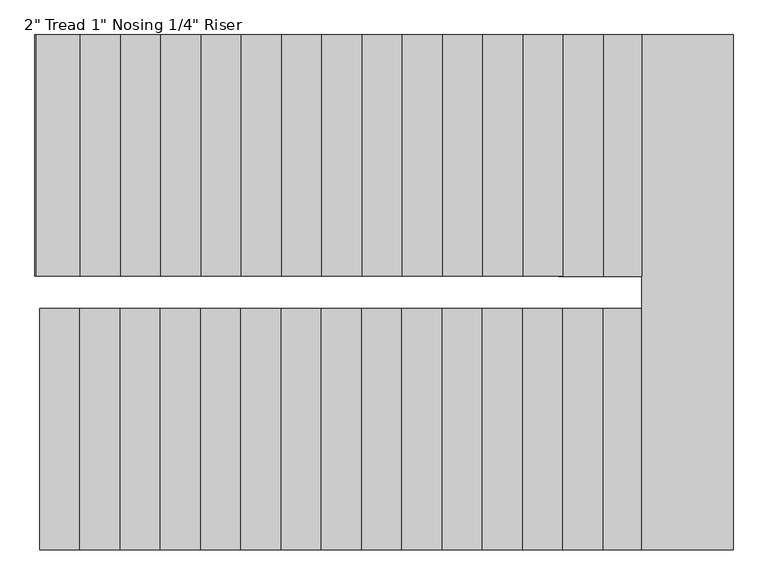
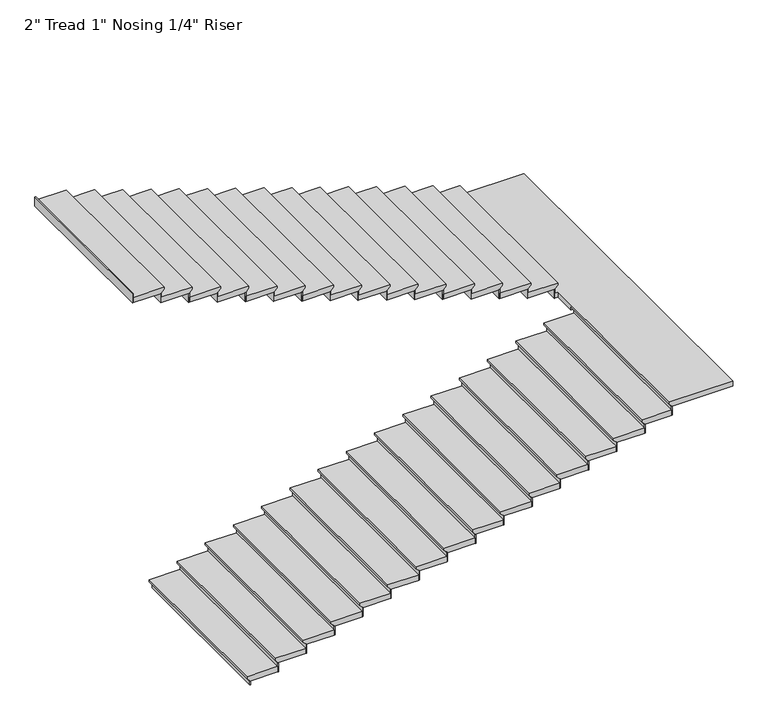
"""IFC4 building model written with IfcOpenShell, lengths in millimetres: stair flight geometry."""

from ifc_helpers import new_model, si_unit, origin, place, context, project, spatial, faceted_brep, source, transform, mapped, element, save


def stair_flight_62363484(model_context):
    return source(origin(), model_context, "Body", "Brep", [
        faceted_brep([(1449.3932247, -2065.2659014, 66.675), (1449.3932247, -2065.2659014, 85.725), (1449.3932247, -541.2659014, 85.725), (1449.3932247, -541.2659014, 66.675), (1474.7932247, -2065.2659014, 41.275), (1474.7932247, -541.2659014, 41.275), (1726.3621616, -2065.2659014, 85.725), (1726.3621616, -541.2659014, 85.725), (1474.7932247, -541.2659014, 34.925), (1726.3621616, -541.2659014, 34.925), (1726.3621616, -2065.2659014, 34.925), (1474.7932247, -2065.2659014, 34.925)], [[[0, 1, 2, 3]], [[4, 0, 3, 5]], [[2, 1, 6, 7]], [[8, 9, 10, 11]], [[2, 7, 9, 8, 5, 3]], [[8, 11, 4, 5]], [[6, 1, 0, 4, 11, 10]], [[7, 6, 10, 9]]]),
        faceted_brep([(1474.7932247, -2065.2659014, 34.925), (1474.7932247, -2065.2659014, 0.0), (1481.1432247, -2065.2659014, 0.0), (1481.1432247, -2065.2659014, 34.925), (1474.7932247, -541.2659014, 34.925), (1481.1432247, -541.2659014, 34.925), (1481.1432247, -541.2659014, 0.0), (1474.7932247, -541.2659014, 0.0)], [[[0, 1, 2, 3]], [[4, 5, 6, 7]], [[1, 0, 4, 7]], [[2, 1, 7, 6]], [[3, 2, 6, 5]], [[0, 3, 5, 4]]]),
        faceted_brep([(1726.3621616, -2065.2659014, 120.65), (1726.3621616, -2065.2659014, 34.925), (1732.7121616, -2065.2659014, 34.925), (1732.7121616, -2065.2659014, 120.65), (1726.3621616, -541.2659014, 120.65), (1732.7121616, -541.2659014, 120.65), (1732.7121616, -541.2659014, 34.925), (1726.3621616, -541.2659014, 34.925)], [[[0, 1, 2, 3]], [[4, 5, 6, 7]], [[1, 0, 4, 7]], [[2, 1, 7, 6]], [[3, 2, 6, 5]], [[0, 3, 5, 4]]]),
        faceted_brep([(1700.9621616, -541.2659014, 171.45), (1700.9621616, -2065.2659014, 171.45), (1980.3621616, -2065.2659014, 171.45), (1980.3621616, -541.2659014, 171.45), (1726.3621616, -541.2659014, 120.65), (1980.3621616, -541.2659014, 120.65), (1980.3621616, -2065.2659014, 120.65), (1726.3621616, -2065.2659014, 120.65), (1726.3621616, -541.2659014, 127.0), (1700.9621616, -541.2659014, 152.4), (1726.3621616, -2065.2659014, 127.0), (1700.9621616, -2065.2659014, 152.4)], [[[0, 1, 2, 3]], [[4, 5, 6, 7]], [[0, 3, 5, 4, 8, 9]], [[4, 7, 10, 8]], [[2, 1, 11, 10, 7, 6]], [[3, 2, 6, 5]], [[11, 1, 0, 9]], [[10, 11, 9, 8]]]),
        faceted_brep([(1980.3621616, -2065.2659014, 206.375), (1980.3621616, -2065.2659014, 120.65), (1986.7121616, -2065.2659014, 120.65), (1986.7121616, -2065.2659014, 206.375), (1980.3621616, -541.2659014, 206.375), (1986.7121616, -541.2659014, 206.375), (1986.7121616, -541.2659014, 120.65), (1980.3621616, -541.2659014, 120.65)], [[[0, 1, 2, 3]], [[4, 5, 6, 7]], [[1, 0, 4, 7]], [[2, 1, 7, 6]], [[3, 2, 6, 5]], [[0, 3, 5, 4]]]),
        faceted_brep([(1954.9621616, -541.2659014, 257.175), (1954.9621616, -2065.2659014, 257.175), (2234.3621616, -2065.2659014, 257.175), (2234.3621616, -541.2659014, 257.175), (1980.3621616, -541.2659014, 206.375), (2234.3621616, -541.2659014, 206.375), (2234.3621616, -2065.2659014, 206.375), (1980.3621616, -2065.2659014, 206.375), (1980.3621616, -541.2659014, 212.725), (1954.9621616, -541.2659014, 238.125), (1980.3621616, -2065.2659014, 212.725), (1954.9621616, -2065.2659014, 238.125)], [[[0, 1, 2, 3]], [[4, 5, 6, 7]], [[0, 3, 5, 4, 8, 9]], [[4, 7, 10, 8]], [[2, 1, 11, 10, 7, 6]], [[3, 2, 6, 5]], [[11, 1, 0, 9]], [[10, 11, 9, 8]]]),
        faceted_brep([(2234.3621616, -2065.2659014, 292.1), (2234.3621616, -2065.2659014, 206.375), (2240.7121616, -2065.2659014, 206.375), (2240.7121616, -2065.2659014, 292.1), (2234.3621616, -541.2659014, 292.1), (2240.7121616, -541.2659014, 292.1), (2240.7121616, -541.2659014, 206.375), (2234.3621616, -541.2659014, 206.375)], [[[0, 1, 2, 3]], [[4, 5, 6, 7]], [[1, 0, 4, 7]], [[2, 1, 7, 6]], [[3, 2, 6, 5]], [[0, 3, 5, 4]]]),
        faceted_brep([(2208.9621616, -541.2659014, 342.9), (2208.9621616, -2065.2659014, 342.9), (2488.3621616, -2065.2659014, 342.9), (2488.3621616, -541.2659014, 342.9), (2234.3621616, -541.2659014, 292.1), (2488.3621616, -541.2659014, 292.1), (2488.3621616, -2065.2659014, 292.1), (2234.3621616, -2065.2659014, 292.1), (2234.3621616, -541.2659014, 298.45), (2208.9621616, -541.2659014, 323.85), (2234.3621616, -2065.2659014, 298.45), (2208.9621616, -2065.2659014, 323.85)], [[[0, 1, 2, 3]], [[4, 5, 6, 7]], [[0, 3, 5, 4, 8, 9]], [[4, 7, 10, 8]], [[2, 1, 11, 10, 7, 6]], [[3, 2, 6, 5]], [[11, 1, 0, 9]], [[10, 11, 9, 8]]]),
        faceted_brep([(2488.3621616, -2065.2659014, 377.825), (2488.3621616, -2065.2659014, 292.1), (2494.7121616, -2065.2659014, 292.1), (2494.7121616, -2065.2659014, 377.825), (2488.3621616, -541.2659014, 377.825), (2494.7121616, -541.2659014, 377.825), (2494.7121616, -541.2659014, 292.1), (2488.3621616, -541.2659014, 292.1)], [[[0, 1, 2, 3]], [[4, 5, 6, 7]], [[1, 0, 4, 7]], [[2, 1, 7, 6]], [[3, 2, 6, 5]], [[0, 3, 5, 4]]]),
        faceted_brep([(2462.9621616, -541.2659014, 428.625), (2462.9621616, -2065.2659014, 428.625), (2742.3621616, -2065.2659014, 428.625), (2742.3621616, -541.2659014, 428.625), (2488.3621616, -541.2659014, 377.825), (2742.3621616, -541.2659014, 377.825), (2742.3621616, -2065.2659014, 377.825), (2488.3621616, -2065.2659014, 377.825), (2488.3621616, -541.2659014, 384.175), (2462.9621616, -541.2659014, 409.575), (2488.3621616, -2065.2659014, 384.175), (2462.9621616, -2065.2659014, 409.575)], [[[0, 1, 2, 3]], [[4, 5, 6, 7]], [[0, 3, 5, 4, 8, 9]], [[4, 7, 10, 8]], [[2, 1, 11, 10, 7, 6]], [[3, 2, 6, 5]], [[11, 1, 0, 9]], [[10, 11, 9, 8]]]),
        faceted_brep([(2742.3621616, -2065.2659014, 463.55), (2742.3621616, -2065.2659014, 377.825), (2748.7121616, -2065.2659014, 377.825), (2748.7121616, -2065.2659014, 463.55), (2742.3621616, -541.2659014, 463.55), (2748.7121616, -541.2659014, 463.55), (2748.7121616, -541.2659014, 377.825), (2742.3621616, -541.2659014, 377.825)], [[[0, 1, 2, 3]], [[4, 5, 6, 7]], [[1, 0, 4, 7]], [[2, 1, 7, 6]], [[3, 2, 6, 5]], [[0, 3, 5, 4]]]),
        faceted_brep([(2716.9621616, -541.2659014, 514.35), (2716.9621616, -2065.2659014, 514.35), (2996.3621616, -2065.2659014, 514.35), (2996.3621616, -541.2659014, 514.35), (2742.3621616, -541.2659014, 463.55), (2996.3621616, -541.2659014, 463.55), (2996.3621616, -2065.2659014, 463.55), (2742.3621616, -2065.2659014, 463.55), (2742.3621616, -541.2659014, 469.9), (2716.9621616, -541.2659014, 495.3), (2742.3621616, -2065.2659014, 469.9), (2716.9621616, -2065.2659014, 495.3)], [[[0, 1, 2, 3]], [[4, 5, 6, 7]], [[0, 3, 5, 4, 8, 9]], [[4, 7, 10, 8]], [[2, 1, 11, 10, 7, 6]], [[3, 2, 6, 5]], [[11, 1, 0, 9]], [[10, 11, 9, 8]]]),
        faceted_brep([(2996.3621616, -2065.2659014, 549.275), (2996.3621616, -2065.2659014, 463.55), (3002.7121616, -2065.2659014, 463.55), (3002.7121616, -2065.2659014, 549.275), (2996.3621616, -541.2659014, 549.275), (3002.7121616, -541.2659014, 549.275), (3002.7121616, -541.2659014, 463.55), (2996.3621616, -541.2659014, 463.55)], [[[0, 1, 2, 3]], [[4, 5, 6, 7]], [[1, 0, 4, 7]], [[2, 1, 7, 6]], [[3, 2, 6, 5]], [[0, 3, 5, 4]]]),
        faceted_brep([(2970.9621616, -541.2659014, 600.075), (2970.9621616, -2065.2659014, 600.075), (3250.3621616, -2065.2659014, 600.075), (3250.3621616, -541.2659014, 600.075), (2996.3621616, -541.2659014, 549.275), (3250.3621616, -541.2659014, 549.275), (3250.3621616, -2065.2659014, 549.275), (2996.3621616, -2065.2659014, 549.275), (2996.3621616, -541.2659014, 555.625), (2970.9621616, -541.2659014, 581.025), (2996.3621616, -2065.2659014, 555.625), (2970.9621616, -2065.2659014, 581.025)], [[[0, 1, 2, 3]], [[4, 5, 6, 7]], [[0, 3, 5, 4, 8, 9]], [[4, 7, 10, 8]], [[2, 1, 11, 10, 7, 6]], [[3, 2, 6, 5]], [[11, 1, 0, 9]], [[10, 11, 9, 8]]]),
        faceted_brep([(3250.3621616, -2065.2659014, 635.0), (3250.3621616, -2065.2659014, 549.275), (3256.7121616, -2065.2659014, 549.275), (3256.7121616, -2065.2659014, 635.0), (3250.3621616, -541.2659014, 635.0), (3256.7121616, -541.2659014, 635.0), (3256.7121616, -541.2659014, 549.275), (3250.3621616, -541.2659014, 549.275)], [[[0, 1, 2, 3]], [[4, 5, 6, 7]], [[1, 0, 4, 7]], [[2, 1, 7, 6]], [[3, 2, 6, 5]], [[0, 3, 5, 4]]]),
        faceted_brep([(3224.9621616, -541.2659014, 685.8), (3224.9621616, -2065.2659014, 685.8), (3504.3621616, -2065.2659014, 685.8), (3504.3621616, -541.2659014, 685.8), (3250.3621616, -541.2659014, 635.0), (3504.3621616, -541.2659014, 635.0), (3504.3621616, -2065.2659014, 635.0), (3250.3621616, -2065.2659014, 635.0), (3250.3621616, -541.2659014, 641.35), (3224.9621616, -541.2659014, 666.75), (3250.3621616, -2065.2659014, 641.35), (3224.9621616, -2065.2659014, 666.75)], [[[0, 1, 2, 3]], [[4, 5, 6, 7]], [[0, 3, 5, 4, 8, 9]], [[4, 7, 10, 8]], [[2, 1, 11, 10, 7, 6]], [[3, 2, 6, 5]], [[11, 1, 0, 9]], [[10, 11, 9, 8]]]),
        faceted_brep([(3504.3621616, -2065.2659014, 720.725), (3504.3621616, -2065.2659014, 635.0), (3510.7121616, -2065.2659014, 635.0), (3510.7121616, -2065.2659014, 720.725), (3504.3621616, -541.2659014, 720.725), (3510.7121616, -541.2659014, 720.725), (3510.7121616, -541.2659014, 635.0), (3504.3621616, -541.2659014, 635.0)], [[[0, 1, 2, 3]], [[4, 5, 6, 7]], [[1, 0, 4, 7]], [[2, 1, 7, 6]], [[3, 2, 6, 5]], [[0, 3, 5, 4]]]),
        faceted_brep([(3478.9621616, -541.2659014, 771.525), (3478.9621616, -2065.2659014, 771.525), (3758.3621616, -2065.2659014, 771.525), (3758.3621616, -541.2659014, 771.525), (3504.3621616, -541.2659014, 720.725), (3758.3621616, -541.2659014, 720.725), (3758.3621616, -2065.2659014, 720.725), (3504.3621616, -2065.2659014, 720.725), (3504.3621616, -541.2659014, 727.075), (3478.9621616, -541.2659014, 752.475), (3504.3621616, -2065.2659014, 727.075), (3478.9621616, -2065.2659014, 752.475)], [[[0, 1, 2, 3]], [[4, 5, 6, 7]], [[0, 3, 5, 4, 8, 9]], [[4, 7, 10, 8]], [[2, 1, 11, 10, 7, 6]], [[3, 2, 6, 5]], [[11, 1, 0, 9]], [[10, 11, 9, 8]]]),
        faceted_brep([(3758.3621616, -2065.2659014, 806.45), (3758.3621616, -2065.2659014, 720.725), (3764.7121616, -2065.2659014, 720.725), (3764.7121616, -2065.2659014, 806.45), (3758.3621616, -541.2659014, 806.45), (3764.7121616, -541.2659014, 806.45), (3764.7121616, -541.2659014, 720.725), (3758.3621616, -541.2659014, 720.725)], [[[0, 1, 2, 3]], [[4, 5, 6, 7]], [[1, 0, 4, 7]], [[2, 1, 7, 6]], [[3, 2, 6, 5]], [[0, 3, 5, 4]]]),
        faceted_brep([(3732.9621616, -541.2659014, 857.25), (3732.9621616, -2065.2659014, 857.25), (4012.3621616, -2065.2659014, 857.25), (4012.3621616, -541.2659014, 857.25), (3758.3621616, -541.2659014, 806.45), (4012.3621616, -541.2659014, 806.45), (4012.3621616, -2065.2659014, 806.45), (3758.3621616, -2065.2659014, 806.45), (3758.3621616, -541.2659014, 812.8), (3732.9621616, -541.2659014, 838.2), (3758.3621616, -2065.2659014, 812.8), (3732.9621616, -2065.2659014, 838.2)], [[[0, 1, 2, 3]], [[4, 5, 6, 7]], [[0, 3, 5, 4, 8, 9]], [[4, 7, 10, 8]], [[2, 1, 11, 10, 7, 6]], [[3, 2, 6, 5]], [[11, 1, 0, 9]], [[10, 11, 9, 8]]]),
        faceted_brep([(4012.3621616, -2065.2659014, 892.175), (4012.3621616, -2065.2659014, 806.45), (4018.7121616, -2065.2659014, 806.45), (4018.7121616, -2065.2659014, 892.175), (4012.3621616, -541.2659014, 892.175), (4018.7121616, -541.2659014, 892.175), (4018.7121616, -541.2659014, 806.45), (4012.3621616, -541.2659014, 806.45)], [[[0, 1, 2, 3]], [[4, 5, 6, 7]], [[1, 0, 4, 7]], [[2, 1, 7, 6]], [[3, 2, 6, 5]], [[0, 3, 5, 4]]]),
        faceted_brep([(3986.9621616, -541.2659014, 942.975), (3986.9621616, -2065.2659014, 942.975), (4266.3621616, -2065.2659014, 942.975), (4266.3621616, -541.2659014, 942.975), (4012.3621616, -541.2659014, 892.175), (4266.3621616, -541.2659014, 892.175), (4266.3621616, -2065.2659014, 892.175), (4012.3621616, -2065.2659014, 892.175), (4012.3621616, -541.2659014, 898.525), (3986.9621616, -541.2659014, 923.925), (4012.3621616, -2065.2659014, 898.525), (3986.9621616, -2065.2659014, 923.925)], [[[0, 1, 2, 3]], [[4, 5, 6, 7]], [[0, 3, 5, 4, 8, 9]], [[4, 7, 10, 8]], [[2, 1, 11, 10, 7, 6]], [[3, 2, 6, 5]], [[11, 1, 0, 9]], [[10, 11, 9, 8]]]),
        faceted_brep([(4266.3621616, -2065.2659014, 977.9), (4266.3621616, -2065.2659014, 892.175), (4272.7121616, -2065.2659014, 892.175), (4272.7121616, -2065.2659014, 977.9), (4266.3621616, -541.2659014, 977.9), (4272.7121616, -541.2659014, 977.9), (4272.7121616, -541.2659014, 892.175), (4266.3621616, -541.2659014, 892.175)], [[[0, 1, 2, 3]], [[4, 5, 6, 7]], [[1, 0, 4, 7]], [[2, 1, 7, 6]], [[3, 2, 6, 5]], [[0, 3, 5, 4]]]),
        faceted_brep([(4240.9621616, -541.2659014, 1028.7), (4240.9621616, -2065.2659014, 1028.7), (4520.3621616, -2065.2659014, 1028.7), (4520.3621616, -541.2659014, 1028.7), (4266.3621616, -541.2659014, 977.9), (4520.3621616, -541.2659014, 977.9), (4520.3621616, -2065.2659014, 977.9), (4266.3621616, -2065.2659014, 977.9), (4266.3621616, -541.2659014, 984.25), (4240.9621616, -541.2659014, 1009.65), (4266.3621616, -2065.2659014, 984.25), (4240.9621616, -2065.2659014, 1009.65)], [[[0, 1, 2, 3]], [[4, 5, 6, 7]], [[0, 3, 5, 4, 8, 9]], [[4, 7, 10, 8]], [[2, 1, 11, 10, 7, 6]], [[3, 2, 6, 5]], [[11, 1, 0, 9]], [[10, 11, 9, 8]]]),
        faceted_brep([(4520.3621616, -2065.2659014, 1063.625), (4520.3621616, -2065.2659014, 977.9), (4526.7121616, -2065.2659014, 977.9), (4526.7121616, -2065.2659014, 1063.625), (4520.3621616, -541.2659014, 1063.625), (4526.7121616, -541.2659014, 1063.625), (4526.7121616, -541.2659014, 977.9), (4520.3621616, -541.2659014, 977.9)], [[[0, 1, 2, 3]], [[4, 5, 6, 7]], [[1, 0, 4, 7]], [[2, 1, 7, 6]], [[3, 2, 6, 5]], [[0, 3, 5, 4]]]),
        faceted_brep([(4494.9621616, -541.2659014, 1114.425), (4494.9621616, -2065.2659014, 1114.425), (4774.3621616, -2065.2659014, 1114.425), (4774.3621616, -541.2659014, 1114.425), (4520.3621616, -541.2659014, 1063.625), (4774.3621616, -541.2659014, 1063.625), (4774.3621616, -2065.2659014, 1063.625), (4520.3621616, -2065.2659014, 1063.625), (4520.3621616, -541.2659014, 1069.975), (4494.9621616, -541.2659014, 1095.375), (4520.3621616, -2065.2659014, 1069.975), (4494.9621616, -2065.2659014, 1095.375)], [[[0, 1, 2, 3]], [[4, 5, 6, 7]], [[0, 3, 5, 4, 8, 9]], [[4, 7, 10, 8]], [[2, 1, 11, 10, 7, 6]], [[3, 2, 6, 5]], [[11, 1, 0, 9]], [[10, 11, 9, 8]]]),
        faceted_brep([(4774.3621616, -2065.2659014, 1149.35), (4774.3621616, -2065.2659014, 1063.625), (4780.7121616, -2065.2659014, 1063.625), (4780.7121616, -2065.2659014, 1149.35), (4774.3621616, -541.2659014, 1149.35), (4780.7121616, -541.2659014, 1149.35), (4780.7121616, -541.2659014, 1063.625), (4774.3621616, -541.2659014, 1063.625)], [[[0, 1, 2, 3]], [[4, 5, 6, 7]], [[1, 0, 4, 7]], [[2, 1, 7, 6]], [[3, 2, 6, 5]], [[0, 3, 5, 4]]]),
        faceted_brep([(4748.9621616, -541.2659014, 1200.15), (4748.9621616, -2065.2659014, 1200.15), (5028.3621616, -2065.2659014, 1200.15), (5028.3621616, -541.2659014, 1200.15), (4774.3621616, -541.2659014, 1149.35), (5028.3621616, -541.2659014, 1149.35), (5028.3621616, -2065.2659014, 1149.35), (4774.3621616, -2065.2659014, 1149.35), (4774.3621616, -541.2659014, 1155.7), (4748.9621616, -541.2659014, 1181.1), (4774.3621616, -2065.2659014, 1155.7), (4748.9621616, -2065.2659014, 1181.1)], [[[0, 1, 2, 3]], [[4, 5, 6, 7]], [[0, 3, 5, 4, 8, 9]], [[4, 7, 10, 8]], [[2, 1, 11, 10, 7, 6]], [[3, 2, 6, 5]], [[11, 1, 0, 9]], [[10, 11, 9, 8]]]),
        faceted_brep([(5028.3621616, -2065.2659014, 1235.075), (5028.3621616, -2065.2659014, 1149.35), (5034.7121616, -2065.2659014, 1149.35), (5034.7121616, -2065.2659014, 1235.075), (5028.3621616, -541.2659014, 1235.075), (5034.7121616, -541.2659014, 1235.075), (5034.7121616, -541.2659014, 1149.35), (5028.3621616, -541.2659014, 1149.35)], [[[0, 1, 2, 3]], [[4, 5, 6, 7]], [[1, 0, 4, 7]], [[2, 1, 7, 6]], [[3, 2, 6, 5]], [[0, 3, 5, 4]]]),
        faceted_brep([(5002.9621616, -541.2659014, 1285.875), (5002.9621616, -2065.2659014, 1285.875), (5272.0669505, -2065.2659014, 1285.875), (5272.0669505, -541.2659014, 1285.875), (5028.3621616, -541.2659014, 1235.075), (5272.0669505, -541.2659014, 1235.075), (5272.0669505, -2065.2659014, 1235.075), (5028.3621616, -2065.2659014, 1235.075), (5028.3621616, -541.2659014, 1241.425), (5002.9621616, -541.2659014, 1266.825), (5028.3621616, -2065.2659014, 1241.425), (5002.9621616, -2065.2659014, 1266.825)], [[[0, 1, 2, 3]], [[4, 5, 6, 7]], [[0, 3, 5, 4, 8, 9]], [[4, 7, 10, 8]], [[2, 1, 11, 10, 7, 6]], [[3, 2, 6, 5]], [[11, 1, 0, 9]], [[10, 11, 9, 8]]]),
        faceted_brep([(5272.0669505, -2065.2659014, 1320.8), (5272.0669505, -2065.2659014, 1235.075), (5278.4169505, -2065.2659014, 1235.075), (5278.4169505, -2065.2659014, 1320.8), (5272.0669505, -541.2659014, 1320.8), (5278.4169505, -541.2659014, 1320.8), (5278.4169505, -541.2659014, 1235.075), (5272.0669505, -541.2659014, 1235.075)], [[[0, 1, 2, 3]], [[4, 5, 6, 7]], [[1, 0, 4, 7]], [[2, 1, 7, 6]], [[3, 2, 6, 5]], [[0, 3, 5, 4]]]),
        faceted_brep([(5221.2669505, -337.9910016, 1371.6), (5246.6669505, -337.9910016, 1371.6), (5246.6669505, -2065.2659014, 1371.6), (5822.2548051, -2065.2659014, 1371.6), (5822.2548051, 1185.9340986, 1371.6), (5221.2669505, 1185.9340986, 1371.6), (5246.6669505, -337.9910016, 1320.8), (5221.2669505, -337.9910016, 1320.8), (5221.2669505, 1185.9340986, 1320.8), (5822.2548051, 1185.9340986, 1320.8), (5822.2548051, -2065.2659014, 1320.8), (5272.0669505, -2065.2659014, 1320.8), (5272.0669505, -541.2659014, 1320.8), (5246.6669505, -541.2659014, 1320.8), (5246.6669505, -541.2659014, 1352.55), (5246.6669505, -2065.2659014, 1352.55), (5272.0669505, -541.2659014, 1327.15), (5272.0669505, -2065.2659014, 1327.15)], [[[0, 1, 2, 3, 4, 5]], [[6, 7, 8, 9, 10, 11, 12, 13]], [[1, 0, 7, 6]], [[2, 1, 6, 13, 14, 15]], [[13, 12, 16, 14]], [[12, 11, 17, 16]], [[3, 2, 15, 17, 11, 10]], [[4, 3, 10, 9]], [[5, 4, 9, 8]], [[0, 5, 8, 7]], [[17, 15, 14, 16]]]),
        faceted_brep([(5221.2669505, 1185.9340986, 1406.525), (5221.2669505, 1185.9340986, 1320.8), (5214.9169505, 1185.9340986, 1320.8), (5214.9169505, 1185.9340986, 1406.525), (5221.2669505, -337.9910016, 1406.525), (5214.9169505, -337.9910016, 1406.525), (5214.9169505, -337.9910016, 1320.8), (5221.2669505, -337.9910016, 1320.8)], [[[0, 1, 2, 3]], [[4, 5, 6, 7]], [[1, 0, 4, 7]], [[2, 1, 7, 6]], [[3, 2, 6, 5]], [[0, 3, 5, 4]]]),
        faceted_brep([(5246.6669505, -337.9910016, 1457.325), (5246.6669505, 1185.9340986, 1457.325), (4977.5621616, 1185.9340986, 1457.325), (4977.5621616, -337.9910016, 1457.325), (5221.2669505, -337.9910016, 1406.525), (4977.5621616, -337.9910016, 1406.525), (4977.5621616, 1185.9340986, 1406.525), (5221.2669505, 1185.9340986, 1406.525), (5221.2669505, -337.9910016, 1412.875), (5246.6669505, -337.9910016, 1438.275), (5221.2669505, 1185.9340986, 1412.875), (5246.6669505, 1185.9340986, 1438.275)], [[[0, 1, 2, 3]], [[4, 5, 6, 7]], [[0, 3, 5, 4, 8, 9]], [[4, 7, 10, 8]], [[2, 1, 11, 10, 7, 6]], [[3, 2, 6, 5]], [[11, 1, 0, 9]], [[10, 11, 9, 8]]]),
        faceted_brep([(4977.5621616, 1185.9340986, 1492.25), (4977.5621616, 1185.9340986, 1406.525), (4971.2121616, 1185.9340986, 1406.525), (4971.2121616, 1185.9340986, 1492.25), (4977.5621616, -337.9910016, 1492.25), (4971.2121616, -337.9910016, 1492.25), (4971.2121616, -337.9910016, 1406.525), (4977.5621616, -337.9910016, 1406.525)], [[[0, 1, 2, 3]], [[4, 5, 6, 7]], [[1, 0, 4, 7]], [[2, 1, 7, 6]], [[3, 2, 6, 5]], [[0, 3, 5, 4]]]),
        faceted_brep([(5002.9621616, -337.9910016, 1543.05), (5002.9621616, 1185.9340986, 1543.05), (4723.5621616, 1185.9340986, 1543.05), (4723.5621616, -337.9910016, 1543.05), (4977.5621616, -337.9910016, 1492.25), (4723.5621616, -337.9910016, 1492.25), (4723.5621616, 1185.9340986, 1492.25), (4977.5621616, 1185.9340986, 1492.25), (4977.5621616, -337.9910016, 1498.6), (5002.9621616, -337.9910016, 1524.0), (4977.5621616, 1185.9340986, 1498.6), (5002.9621616, 1185.9340986, 1524.0)], [[[0, 1, 2, 3]], [[4, 5, 6, 7]], [[0, 3, 5, 4, 8, 9]], [[4, 7, 10, 8]], [[2, 1, 11, 10, 7, 6]], [[3, 2, 6, 5]], [[11, 1, 0, 9]], [[10, 11, 9, 8]]]),
        faceted_brep([(4723.5621616, 1185.9340986, 1577.975), (4723.5621616, 1185.9340986, 1492.25), (4717.2121616, 1185.9340986, 1492.25), (4717.2121616, 1185.9340986, 1577.975), (4723.5621616, -337.9910016, 1577.975), (4717.2121616, -337.9910016, 1577.975), (4717.2121616, -337.9910016, 1492.25), (4723.5621616, -337.9910016, 1492.25)], [[[0, 1, 2, 3]], [[4, 5, 6, 7]], [[1, 0, 4, 7]], [[2, 1, 7, 6]], [[3, 2, 6, 5]], [[0, 3, 5, 4]]]),
        faceted_brep([(4748.9621616, -337.9910016, 1628.775), (4748.9621616, 1185.9340986, 1628.775), (4469.5621616, 1185.9340986, 1628.775), (4469.5621616, -337.9910016, 1628.775), (4723.5621616, -337.9910016, 1577.975), (4469.5621616, -337.9910016, 1577.975), (4469.5621616, 1185.9340986, 1577.975), (4723.5621616, 1185.9340986, 1577.975), (4723.5621616, -337.9910016, 1584.325), (4748.9621616, -337.9910016, 1609.725), (4723.5621616, 1185.9340986, 1584.325), (4748.9621616, 1185.9340986, 1609.725)], [[[0, 1, 2, 3]], [[4, 5, 6, 7]], [[0, 3, 5, 4, 8, 9]], [[4, 7, 10, 8]], [[2, 1, 11, 10, 7, 6]], [[3, 2, 6, 5]], [[11, 1, 0, 9]], [[10, 11, 9, 8]]]),
        faceted_brep([(4469.5621616, 1185.9340986, 1663.7), (4469.5621616, 1185.9340986, 1577.975), (4463.2121616, 1185.9340986, 1577.975), (4463.2121616, 1185.9340986, 1663.7), (4469.5621616, -337.9910016, 1663.7), (4463.2121616, -337.9910016, 1663.7), (4463.2121616, -337.9910016, 1577.975), (4469.5621616, -337.9910016, 1577.975)], [[[0, 1, 2, 3]], [[4, 5, 6, 7]], [[1, 0, 4, 7]], [[2, 1, 7, 6]], [[3, 2, 6, 5]], [[0, 3, 5, 4]]]),
        faceted_brep([(4494.9621616, -337.9910016, 1714.5), (4494.9621616, 1185.9340986, 1714.5), (4215.5621616, 1185.9340986, 1714.5), (4215.5621616, -337.9910016, 1714.5), (4469.5621616, -337.9910016, 1663.7), (4215.5621616, -337.9910016, 1663.7), (4215.5621616, 1185.9340986, 1663.7), (4469.5621616, 1185.9340986, 1663.7), (4469.5621616, -337.9910016, 1670.05), (4494.9621616, -337.9910016, 1695.45), (4469.5621616, 1185.9340986, 1670.05), (4494.9621616, 1185.9340986, 1695.45)], [[[0, 1, 2, 3]], [[4, 5, 6, 7]], [[0, 3, 5, 4, 8, 9]], [[4, 7, 10, 8]], [[2, 1, 11, 10, 7, 6]], [[3, 2, 6, 5]], [[11, 1, 0, 9]], [[10, 11, 9, 8]]]),
        faceted_brep([(4215.5621616, 1185.9340986, 1749.425), (4215.5621616, 1185.9340986, 1663.7), (4209.2121616, 1185.9340986, 1663.7), (4209.2121616, 1185.9340986, 1749.425), (4215.5621616, -337.9910016, 1749.425), (4209.2121616, -337.9910016, 1749.425), (4209.2121616, -337.9910016, 1663.7), (4215.5621616, -337.9910016, 1663.7)], [[[0, 1, 2, 3]], [[4, 5, 6, 7]], [[1, 0, 4, 7]], [[2, 1, 7, 6]], [[3, 2, 6, 5]], [[0, 3, 5, 4]]]),
        faceted_brep([(4240.9621616, -337.9910016, 1800.225), (4240.9621616, 1185.9340986, 1800.225), (3961.5621616, 1185.9340986, 1800.225), (3961.5621616, -337.9910016, 1800.225), (4215.5621616, -337.9910016, 1749.425), (3961.5621616, -337.9910016, 1749.425), (3961.5621616, 1185.9340986, 1749.425), (4215.5621616, 1185.9340986, 1749.425), (4215.5621616, -337.9910016, 1755.775), (4240.9621616, -337.9910016, 1781.175), (4215.5621616, 1185.9340986, 1755.775), (4240.9621616, 1185.9340986, 1781.175)], [[[0, 1, 2, 3]], [[4, 5, 6, 7]], [[0, 3, 5, 4, 8, 9]], [[4, 7, 10, 8]], [[2, 1, 11, 10, 7, 6]], [[3, 2, 6, 5]], [[11, 1, 0, 9]], [[10, 11, 9, 8]]]),
        faceted_brep([(3961.5621616, 1185.9340986, 1835.15), (3961.5621616, 1185.9340986, 1749.425), (3955.2121616, 1185.9340986, 1749.425), (3955.2121616, 1185.9340986, 1835.15), (3961.5621616, -337.9910016, 1835.15), (3955.2121616, -337.9910016, 1835.15), (3955.2121616, -337.9910016, 1749.425), (3961.5621616, -337.9910016, 1749.425)], [[[0, 1, 2, 3]], [[4, 5, 6, 7]], [[1, 0, 4, 7]], [[2, 1, 7, 6]], [[3, 2, 6, 5]], [[0, 3, 5, 4]]]),
        faceted_brep([(3986.9621616, -337.9910016, 1885.95), (3986.9621616, 1185.9340986, 1885.95), (3707.5621616, 1185.9340986, 1885.95), (3707.5621616, -337.9910016, 1885.95), (3961.5621616, -337.9910016, 1835.15), (3707.5621616, -337.9910016, 1835.15), (3707.5621616, 1185.9340986, 1835.15), (3961.5621616, 1185.9340986, 1835.15), (3961.5621616, -337.9910016, 1841.5), (3986.9621616, -337.9910016, 1866.9), (3961.5621616, 1185.9340986, 1841.5), (3986.9621616, 1185.9340986, 1866.9)], [[[0, 1, 2, 3]], [[4, 5, 6, 7]], [[0, 3, 5, 4, 8, 9]], [[4, 7, 10, 8]], [[2, 1, 11, 10, 7, 6]], [[3, 2, 6, 5]], [[11, 1, 0, 9]], [[10, 11, 9, 8]]]),
        faceted_brep([(3707.5621616, 1185.9340986, 1920.875), (3707.5621616, 1185.9340986, 1835.15), (3701.2121616, 1185.9340986, 1835.15), (3701.2121616, 1185.9340986, 1920.875), (3707.5621616, -337.9910016, 1920.875), (3701.2121616, -337.9910016, 1920.875), (3701.2121616, -337.9910016, 1835.15), (3707.5621616, -337.9910016, 1835.15)], [[[0, 1, 2, 3]], [[4, 5, 6, 7]], [[1, 0, 4, 7]], [[2, 1, 7, 6]], [[3, 2, 6, 5]], [[0, 3, 5, 4]]]),
        faceted_brep([(3732.9621616, -337.9910016, 1971.675), (3732.9621616, 1185.9340986, 1971.675), (3453.5621616, 1185.9340986, 1971.675), (3453.5621616, -337.9910016, 1971.675), (3707.5621616, -337.9910016, 1920.875), (3453.5621616, -337.9910016, 1920.875), (3453.5621616, 1185.9340986, 1920.875), (3707.5621616, 1185.9340986, 1920.875), (3707.5621616, -337.9910016, 1927.225), (3732.9621616, -337.9910016, 1952.625), (3707.5621616, 1185.9340986, 1927.225), (3732.9621616, 1185.9340986, 1952.625)], [[[0, 1, 2, 3]], [[4, 5, 6, 7]], [[0, 3, 5, 4, 8, 9]], [[4, 7, 10, 8]], [[2, 1, 11, 10, 7, 6]], [[3, 2, 6, 5]], [[11, 1, 0, 9]], [[10, 11, 9, 8]]]),
        faceted_brep([(3453.5621616, 1185.9340986, 2006.6), (3453.5621616, 1185.9340986, 1920.875), (3447.2121616, 1185.9340986, 1920.875), (3447.2121616, 1185.9340986, 2006.6), (3453.5621616, -337.9910016, 2006.6), (3447.2121616, -337.9910016, 2006.6), (3447.2121616, -337.9910016, 1920.875), (3453.5621616, -337.9910016, 1920.875)], [[[0, 1, 2, 3]], [[4, 5, 6, 7]], [[1, 0, 4, 7]], [[2, 1, 7, 6]], [[3, 2, 6, 5]], [[0, 3, 5, 4]]]),
        faceted_brep([(3478.9621616, -337.9910016, 2057.4), (3478.9621616, 1185.9340986, 2057.4), (3199.5621616, 1185.9340986, 2057.4), (3199.5621616, -337.9910016, 2057.4), (3453.5621616, -337.9910016, 2006.6), (3199.5621616, -337.9910016, 2006.6), (3199.5621616, 1185.9340986, 2006.6), (3453.5621616, 1185.9340986, 2006.6), (3453.5621616, -337.9910016, 2012.95), (3478.9621616, -337.9910016, 2038.35), (3453.5621616, 1185.9340986, 2012.95), (3478.9621616, 1185.9340986, 2038.35)], [[[0, 1, 2, 3]], [[4, 5, 6, 7]], [[0, 3, 5, 4, 8, 9]], [[4, 7, 10, 8]], [[2, 1, 11, 10, 7, 6]], [[3, 2, 6, 5]], [[11, 1, 0, 9]], [[10, 11, 9, 8]]]),
        faceted_brep([(3199.5621616, 1185.9340986, 2092.325), (3199.5621616, 1185.9340986, 2006.6), (3193.2121616, 1185.9340986, 2006.6), (3193.2121616, 1185.9340986, 2092.325), (3199.5621616, -337.9910016, 2092.325), (3193.2121616, -337.9910016, 2092.325), (3193.2121616, -337.9910016, 2006.6), (3199.5621616, -337.9910016, 2006.6)], [[[0, 1, 2, 3]], [[4, 5, 6, 7]], [[1, 0, 4, 7]], [[2, 1, 7, 6]], [[3, 2, 6, 5]], [[0, 3, 5, 4]]]),
        faceted_brep([(3224.9621616, -337.9910016, 2143.125), (3224.9621616, 1185.9340986, 2143.125), (2945.5621616, 1185.9340986, 2143.125), (2945.5621616, -337.9910016, 2143.125), (3199.5621616, -337.9910016, 2092.325), (2945.5621616, -337.9910016, 2092.325), (2945.5621616, 1185.9340986, 2092.325), (3199.5621616, 1185.9340986, 2092.325), (3199.5621616, -337.9910016, 2098.675), (3224.9621616, -337.9910016, 2124.075), (3199.5621616, 1185.9340986, 2098.675), (3224.9621616, 1185.9340986, 2124.075)], [[[0, 1, 2, 3]], [[4, 5, 6, 7]], [[0, 3, 5, 4, 8, 9]], [[4, 7, 10, 8]], [[2, 1, 11, 10, 7, 6]], [[3, 2, 6, 5]], [[11, 1, 0, 9]], [[10, 11, 9, 8]]]),
        faceted_brep([(2945.5621616, 1185.9340986, 2178.05), (2945.5621616, 1185.9340986, 2092.325), (2939.2121616, 1185.9340986, 2092.325), (2939.2121616, 1185.9340986, 2178.05), (2945.5621616, -337.9910016, 2178.05), (2939.2121616, -337.9910016, 2178.05), (2939.2121616, -337.9910016, 2092.325), (2945.5621616, -337.9910016, 2092.325)], [[[0, 1, 2, 3]], [[4, 5, 6, 7]], [[1, 0, 4, 7]], [[2, 1, 7, 6]], [[3, 2, 6, 5]], [[0, 3, 5, 4]]]),
        faceted_brep([(2970.9621616, -337.9910016, 2228.85), (2970.9621616, 1185.9340986, 2228.85), (2691.5621616, 1185.9340986, 2228.85), (2691.5621616, -337.9910016, 2228.85), (2945.5621616, -337.9910016, 2178.05), (2691.5621616, -337.9910016, 2178.05), (2691.5621616, 1185.9340986, 2178.05), (2945.5621616, 1185.9340986, 2178.05), (2945.5621616, -337.9910016, 2184.4), (2970.9621616, -337.9910016, 2209.8), (2945.5621616, 1185.9340986, 2184.4), (2970.9621616, 1185.9340986, 2209.8)], [[[0, 1, 2, 3]], [[4, 5, 6, 7]], [[0, 3, 5, 4, 8, 9]], [[4, 7, 10, 8]], [[2, 1, 11, 10, 7, 6]], [[3, 2, 6, 5]], [[11, 1, 0, 9]], [[10, 11, 9, 8]]]),
        faceted_brep([(2691.5621616, 1185.9340986, 2263.775), (2691.5621616, 1185.9340986, 2178.05), (2685.2121616, 1185.9340986, 2178.05), (2685.2121616, 1185.9340986, 2263.775), (2691.5621616, -337.9910016, 2263.775), (2685.2121616, -337.9910016, 2263.775), (2685.2121616, -337.9910016, 2178.05), (2691.5621616, -337.9910016, 2178.05)], [[[0, 1, 2, 3]], [[4, 5, 6, 7]], [[1, 0, 4, 7]], [[2, 1, 7, 6]], [[3, 2, 6, 5]], [[0, 3, 5, 4]]]),
        faceted_brep([(2716.9621616, -337.9910016, 2314.575), (2716.9621616, 1185.9340986, 2314.575), (2437.5621616, 1185.9340986, 2314.575), (2437.5621616, -337.9910016, 2314.575), (2691.5621616, -337.9910016, 2263.775), (2437.5621616, -337.9910016, 2263.775), (2437.5621616, 1185.9340986, 2263.775), (2691.5621616, 1185.9340986, 2263.775), (2691.5621616, -337.9910016, 2270.125), (2716.9621616, -337.9910016, 2295.525), (2691.5621616, 1185.9340986, 2270.125), (2716.9621616, 1185.9340986, 2295.525)], [[[0, 1, 2, 3]], [[4, 5, 6, 7]], [[0, 3, 5, 4, 8, 9]], [[4, 7, 10, 8]], [[2, 1, 11, 10, 7, 6]], [[3, 2, 6, 5]], [[11, 1, 0, 9]], [[10, 11, 9, 8]]]),
        faceted_brep([(2437.5621616, 1185.9340986, 2349.5), (2437.5621616, 1185.9340986, 2263.775), (2431.2121616, 1185.9340986, 2263.775), (2431.2121616, 1185.9340986, 2349.5), (2437.5621616, -337.9910016, 2349.5), (2431.2121616, -337.9910016, 2349.5), (2431.2121616, -337.9910016, 2263.775), (2437.5621616, -337.9910016, 2263.775)], [[[0, 1, 2, 3]], [[4, 5, 6, 7]], [[1, 0, 4, 7]], [[2, 1, 7, 6]], [[3, 2, 6, 5]], [[0, 3, 5, 4]]]),
        faceted_brep([(2462.9621616, -337.9910016, 2400.3), (2462.9621616, 1185.9340986, 2400.3), (2183.5621616, 1185.9340986, 2400.3), (2183.5621616, -337.9910016, 2400.3), (2437.5621616, -337.9910016, 2349.5), (2183.5621616, -337.9910016, 2349.5), (2183.5621616, 1185.9340986, 2349.5), (2437.5621616, 1185.9340986, 2349.5), (2437.5621616, -337.9910016, 2355.85), (2462.9621616, -337.9910016, 2381.25), (2437.5621616, 1185.9340986, 2355.85), (2462.9621616, 1185.9340986, 2381.25)], [[[0, 1, 2, 3]], [[4, 5, 6, 7]], [[0, 3, 5, 4, 8, 9]], [[4, 7, 10, 8]], [[2, 1, 11, 10, 7, 6]], [[3, 2, 6, 5]], [[11, 1, 0, 9]], [[10, 11, 9, 8]]]),
        faceted_brep([(2183.5621616, 1185.9340986, 2435.225), (2183.5621616, 1185.9340986, 2349.5), (2177.2121616, 1185.9340986, 2349.5), (2177.2121616, 1185.9340986, 2435.225), (2183.5621616, -337.9910016, 2435.225), (2177.2121616, -337.9910016, 2435.225), (2177.2121616, -337.9910016, 2349.5), (2183.5621616, -337.9910016, 2349.5)], [[[0, 1, 2, 3]], [[4, 5, 6, 7]], [[1, 0, 4, 7]], [[2, 1, 7, 6]], [[3, 2, 6, 5]], [[0, 3, 5, 4]]]),
        faceted_brep([(2208.9621616, -337.9910016, 2486.025), (2208.9621616, 1185.9340986, 2486.025), (1929.5621616, 1185.9340986, 2486.025), (1929.5621616, -337.9910016, 2486.025), (2183.5621616, -337.9910016, 2435.225), (1929.5621616, -337.9910016, 2435.225), (1929.5621616, 1185.9340986, 2435.225), (2183.5621616, 1185.9340986, 2435.225), (2183.5621616, -337.9910016, 2441.575), (2208.9621616, -337.9910016, 2466.975), (2183.5621616, 1185.9340986, 2441.575), (2208.9621616, 1185.9340986, 2466.975)], [[[0, 1, 2, 3]], [[4, 5, 6, 7]], [[0, 3, 5, 4, 8, 9]], [[4, 7, 10, 8]], [[2, 1, 11, 10, 7, 6]], [[3, 2, 6, 5]], [[11, 1, 0, 9]], [[10, 11, 9, 8]]]),
        faceted_brep([(1929.5621616, 1185.9340986, 2520.95), (1929.5621616, 1185.9340986, 2435.225), (1923.2121616, 1185.9340986, 2435.225), (1923.2121616, 1185.9340986, 2520.95), (1929.5621616, -337.9910016, 2520.95), (1923.2121616, -337.9910016, 2520.95), (1923.2121616, -337.9910016, 2435.225), (1929.5621616, -337.9910016, 2435.225)], [[[0, 1, 2, 3]], [[4, 5, 6, 7]], [[1, 0, 4, 7]], [[2, 1, 7, 6]], [[3, 2, 6, 5]], [[0, 3, 5, 4]]]),
        faceted_brep([(1954.9621616, -337.9910016, 2571.75), (1954.9621616, 1185.9340986, 2571.75), (1675.5621616, 1185.9340986, 2571.75), (1675.5621616, -337.9910016, 2571.75), (1929.5621616, -337.9910016, 2520.95), (1675.5621616, -337.9910016, 2520.95), (1675.5621616, 1185.9340986, 2520.95), (1929.5621616, 1185.9340986, 2520.95), (1929.5621616, -337.9910016, 2527.3), (1954.9621616, -337.9910016, 2552.7), (1929.5621616, 1185.9340986, 2527.3), (1954.9621616, 1185.9340986, 2552.7)], [[[0, 1, 2, 3]], [[4, 5, 6, 7]], [[0, 3, 5, 4, 8, 9]], [[4, 7, 10, 8]], [[2, 1, 11, 10, 7, 6]], [[3, 2, 6, 5]], [[11, 1, 0, 9]], [[10, 11, 9, 8]]]),
        faceted_brep([(1675.5621616, 1185.9340986, 2606.675), (1675.5621616, 1185.9340986, 2520.95), (1669.2121616, 1185.9340986, 2520.95), (1669.2121616, 1185.9340986, 2606.675), (1675.5621616, -337.9910016, 2606.675), (1669.2121616, -337.9910016, 2606.675), (1669.2121616, -337.9910016, 2520.95), (1675.5621616, -337.9910016, 2520.95)], [[[0, 1, 2, 3]], [[4, 5, 6, 7]], [[1, 0, 4, 7]], [[2, 1, 7, 6]], [[3, 2, 6, 5]], [[0, 3, 5, 4]]]),
        faceted_brep([(1423.9932247, 1185.9340986, 2692.4), (1423.9932247, 1185.9340986, 2606.675), (1417.6432247, 1185.9340986, 2606.675), (1417.6432247, 1185.9340986, 2692.4), (1423.9932247, -337.9910016, 2692.4), (1417.6432247, -337.9910016, 2692.4), (1417.6432247, -337.9910016, 2606.675), (1423.9932247, -337.9910016, 2606.675)], [[[0, 1, 2, 3]], [[4, 5, 6, 7]], [[1, 0, 4, 7]], [[2, 1, 7, 6]], [[3, 2, 6, 5]], [[0, 3, 5, 4]]]),
        faceted_brep([(1700.9621616, -337.9910016, 2657.475), (1700.9621616, 1185.9340986, 2657.475), (1423.9932247, 1185.9340986, 2657.475), (1423.9932247, -337.9910016, 2657.475), (1675.5621616, -337.9910016, 2606.675), (1423.9932247, -337.9910016, 2606.675), (1423.9932247, 1185.9340986, 2606.675), (1675.5621616, 1185.9340986, 2606.675), (1675.5621616, -337.9910016, 2613.025), (1700.9621616, -337.9910016, 2638.425), (1675.5621616, 1185.9340986, 2613.025), (1700.9621616, 1185.9340986, 2638.425)], [[[0, 1, 2, 3]], [[4, 5, 6, 7]], [[0, 3, 5, 4, 8, 9]], [[4, 7, 10, 8]], [[2, 1, 11, 10, 7, 6]], [[3, 2, 6, 5]], [[11, 1, 0, 9]], [[10, 11, 9, 8]]]),
    ])


if __name__ == "__main__":
    model = new_model("IFC4")
    model_context = context("Model", 3, world=origin())
    ifc_project = project(units=[si_unit("LENGTHUNIT", "METRE", prefix="MILLI")], contexts=[model_context])
    site = spatial("IfcSite", under=ifc_project)
    building = spatial("IfcBuilding", under=site)
    placement = place(None, origin())
    stair_flight_shape = stair_flight_62363484(model_context)
    element("IfcStairFlight", 1, ObjectType="2\" Tread 1\" Nosing 1/4\" Riser", at=placement, inside=building, context=model_context, shape_type="MappedRepresentation", body=[
        mapped(stair_flight_shape, transform((0.0, 0.0, 0.0), x_axis=(1.0, 0.0, 0.0), y_axis=(0.0, 1.0, 0.0), z_axis=(0.0, 0.0, 1.0))),
    ])
    save(model, "model.ifc")
